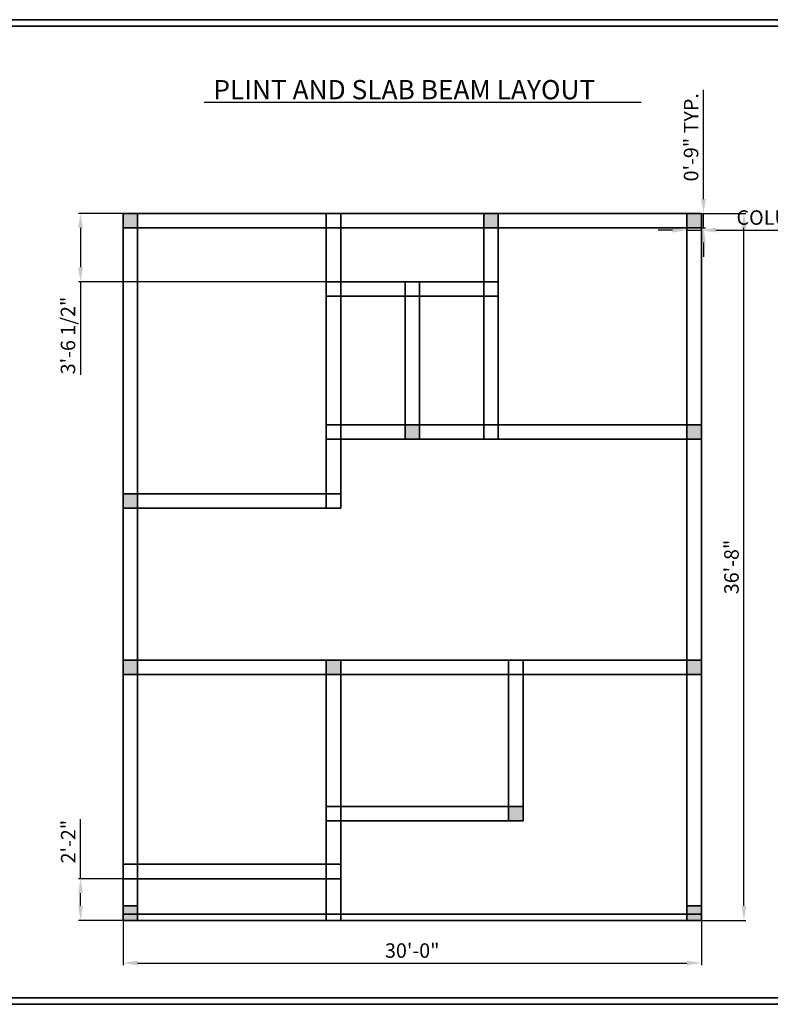
# Model space of a CAD drawing. Units: inches. Extents: x 2436 to 3928, y 1526 to 2149.
# Tile 5 of 6: x 2903 to 3371, y 1526 to 2138. Entities that reach past the tile are written whole.
import ezdxf

# ---------------------------------------------------------------- set-up
doc = ezdxf.new("R2010")
doc.units = ezdxf.units.IN
for name, color, linetype, lineweight in [('G-ANNO-TEXT', 7, 'Continuous', 25), ('G-ANNO-TTLB', 7, 'Continuous', 35), ('S-ANNO-DIMS', 2, 'Continuous', 18), ('S-BEAM', 7, 'Continuous', 35), ('S-COLS', 1, 'Continuous', 35), ('S-COLS-PATT', 1, 'Continuous', 13)]:
    doc.layers.add(name, color=color, linetype=linetype, lineweight=lineweight)
doc.styles.get("Standard").update_dxf_attribs({"font": 'arial.ttf'})
doc.dimstyles.new('ISO-25', dxfattribs={"dimtxt": 9, "dimasz": 9, "dimexe": 1.25, "dimexo": 0.625, "dimgap": 2, "dimtad": 1, "dimdec": 1, "dimlunit": 4, "dimtxsty": 'Standard', "dimcen": 2.5, "dimadec": 0, "dimazin": 0, "dimtfac": 1, "dimtdec": 1, "dimtmove": 0, "dimatfit": 3, "dimfxl": 1, "dimarcsym": 0})

# ---------------------------------------------------------------- blocks, each defined once
blk = doc.blocks.new('COL-9x9-PLAN')
h = blk.add_hatch(color=256)
h.dxf.hatch_style = 1
h.paths.add_polyline_path([(9, 0), (9, 9), (0, 9), (0, 0)])
blk.add_lwpolyline([(0, 9), (9, 9), (9, 0), (0, 0)], close=True)
blk = doc.blocks.new('*D30')
at = {"layer": 'Defpoints', "color": 0, "transparency": 16777216}
for p in [(3318.67, 2008.79), (3327.67, 2008.79), (3327.67, 2007.44)]:
    blk.add_point(p, dxfattribs=at)
at = {"layer": 'S-ANNO-DIMS', "color": 0, "lineweight": -2, "transparency": 16777216}
for p, q in [((3309.67, 2007.44), (3300.67, 2007.44)), ((3318.67, 2008.16), (3318.67, 2006.19)), ((3318.67, 2007.44), (3327.67, 2007.44)), ((3327.67, 2008.16), (3327.67, 2006.19)), ((3336.67, 2007.44), (3462.4, 2007.44))]:
    blk.add_line(p, q, dxfattribs=at)
at = {"layer": 'S-ANNO-DIMS', "color": 0, "transparency": 16777216}
for points in [[(3309.67, 2008.94), (3309.67, 2005.94), (3318.67, 2007.44)], [(3336.67, 2008.94), (3336.67, 2005.94), (3327.67, 2007.44)]]:
    blk.add_solid(points, dxfattribs=at)
at = {"layer": 'S-ANNO-DIMS', "color": 0, "transparency": 16777216, "insert": (3404.03, 2014.1), "char_height": 9, "attachment_point": 5}
blk.add_mtext('COLUMN 0\'-9" TYP.', dxfattribs=at)
blk = doc.blocks.new('*D31')
at = {"layer": 'Defpoints', "color": 0, "transparency": 16777216}
for p in [(3327.67, 2017.79), (3329.02, 2017.79), (3327.67, 2008.79)]:
    blk.add_point(p, dxfattribs=at)
at = {"layer": 'S-ANNO-DIMS', "color": 0, "lineweight": -2, "transparency": 16777216}
for p, q in [((3329.02, 2026.79), (3329.02, 2094.65)), ((3328.29, 2017.79), (3330.27, 2017.79)), ((3329.02, 2008.79), (3329.02, 2017.79)), ((3328.29, 2008.79), (3330.27, 2008.79)), ((3329.02, 1999.79), (3329.02, 1990.79))]:
    blk.add_line(p, q, dxfattribs=at)
at = {"layer": 'S-ANNO-DIMS', "color": 0, "transparency": 16777216}
for points in [[(3327.52, 2026.79), (3330.52, 2026.79), (3329.02, 2017.79)], [(3327.52, 1999.79), (3330.52, 1999.79), (3329.02, 2008.79)]]:
    blk.add_solid(points, dxfattribs=at)
at = {"layer": 'S-ANNO-DIMS', "color": 0, "transparency": 16777216, "insert": (3322.42, 2065.22), "char_height": 9, "attachment_point": 5, "rotation": 90}
blk.add_mtext('0\'-9" TYP.', dxfattribs=at)
blk = doc.blocks.new('*D74')
at = {"layer": 'Defpoints', "color": 0, "transparency": 16777216}
for p in [(2967.67, 1577.79), (3327.67, 1577.79), (3327.67, 1551.29)]:
    blk.add_point(p, dxfattribs=at)
at = {"layer": 'S-ANNO-DIMS', "color": 0, "lineweight": -2, "transparency": 16777216}
for p, q in [((2967.67, 1577.16), (2967.67, 1550.04)), ((3327.67, 1577.16), (3327.67, 1550.04)), ((2976.67, 1551.29), (3318.67, 1551.29))]:
    blk.add_line(p, q, dxfattribs=at)
at = {"layer": 'S-ANNO-DIMS', "color": 0, "transparency": 16777216}
for points in [[(2976.67, 1552.79), (2976.67, 1549.79), (2967.67, 1551.29)], [(3318.67, 1552.79), (3318.67, 1549.79), (3327.67, 1551.29)]]:
    blk.add_solid(points, dxfattribs=at)
at = {"layer": 'S-ANNO-DIMS', "color": 0, "transparency": 16777216, "insert": (3147.67, 1557.89), "char_height": 9, "attachment_point": 5}
blk.add_mtext('30\'-0"', dxfattribs=at)
blk = doc.blocks.new('*D75')
at = {"layer": 'Defpoints', "color": 0, "transparency": 16777216}
for p in [(3327.67, 2017.79), (3354.17, 2017.79), (3327.67, 1577.79)]:
    blk.add_point(p, dxfattribs=at)
at = {"layer": 'S-ANNO-DIMS', "color": 0, "lineweight": -2, "transparency": 16777216}
for p, q in [((3328.29, 2017.79), (3355.42, 2017.79)), ((3354.17, 1586.79), (3354.17, 2008.79)), ((3328.29, 1577.79), (3355.42, 1577.79))]:
    blk.add_line(p, q, dxfattribs=at)
at = {"layer": 'S-ANNO-DIMS', "color": 0, "transparency": 16777216}
for points in [[(3352.67, 2008.79), (3355.67, 2008.79), (3354.17, 2017.79)], [(3352.67, 1586.79), (3355.67, 1586.79), (3354.17, 1577.79)]]:
    blk.add_solid(points, dxfattribs=at)
at = {"layer": 'S-ANNO-DIMS', "color": 0, "transparency": 16777216, "insert": (3347.57, 1797.79), "char_height": 9, "attachment_point": 5, "rotation": 90}
blk.add_mtext('36\'-8"', dxfattribs=at)
blk = doc.blocks.new('*D76')
at = {"layer": 'Defpoints', "color": 0, "transparency": 16777216}
for p in [(3094.17, 2017.79), (2941.17, 1975.29), (3094.17, 1975.29)]:
    blk.add_point(p, dxfattribs=at)
at = {"layer": 'S-ANNO-DIMS', "color": 0, "lineweight": -2, "transparency": 16777216}
for p, q in [((3093.54, 2017.79), (2939.92, 2017.79)), ((2941.17, 2008.79), (2941.17, 1984.29)), ((3093.54, 1975.29), (2939.92, 1975.29)), ((2941.17, 1975.29), (2941.17, 1917.4))]:
    blk.add_line(p, q, dxfattribs=at)
at = {"layer": 'S-ANNO-DIMS', "color": 0, "transparency": 16777216}
for points in [[(2939.67, 2008.79), (2942.67, 2008.79), (2941.17, 2017.79)], [(2939.67, 1984.29), (2942.67, 1984.29), (2941.17, 1975.29)]]:
    blk.add_solid(points, dxfattribs=at)
at = {"layer": 'S-ANNO-DIMS', "color": 0, "transparency": 16777216, "insert": (2934.51, 1941.84), "char_height": 9, "attachment_point": 5, "rotation": 90}
blk.add_mtext('3\'-6 1/2"', dxfattribs=at)
blk = doc.blocks.new('*D77')
at = {"layer": 'Defpoints', "color": 0, "transparency": 16777216}
for p in [(2941.17, 1603.79), (2967.67, 1603.79), (2967.67, 1577.79)]:
    blk.add_point(p, dxfattribs=at)
at = {"layer": 'S-ANNO-DIMS', "color": 0, "lineweight": -2, "transparency": 16777216}
for p, q in [((2941.17, 1603.79), (2941.17, 1640.87)), ((2967.04, 1603.79), (2939.92, 1603.79)), ((2941.17, 1586.79), (2941.17, 1594.79)), ((2967.04, 1577.79), (2939.92, 1577.79))]:
    blk.add_line(p, q, dxfattribs=at)
at = {"layer": 'S-ANNO-DIMS', "color": 0, "transparency": 16777216}
for points in [[(2939.67, 1594.79), (2942.67, 1594.79), (2941.17, 1603.79)], [(2939.67, 1586.79), (2942.67, 1586.79), (2941.17, 1577.79)]]:
    blk.add_solid(points, dxfattribs=at)
at = {"layer": 'S-ANNO-DIMS', "color": 0, "transparency": 16777216, "insert": (2934.65, 1626.83), "char_height": 9, "attachment_point": 5, "rotation": 90}
blk.add_mtext('2\'-2"', dxfattribs=at)

msp = doc.modelspace()

# ---------------------------------------------------------------- hatches: boundary and pattern name
at = {"layer": 'S-COLS-PATT'}
h = msp.add_hatch(color=256, dxfattribs=at)
h.dxf.hatch_style = 1
h.paths.add_polyline_path([(3327.67, 1739.79), (3318.67, 1739.79), (3318.67, 1730.79), (3327.67, 1730.79)])

# ---------------------------------------------------------------- linework, layer by layer
at = {"layer": 'G-ANNO-TEXT'}
msp.add_line((3018.04, 2087.13), (3290.21, 2087.13), dxfattribs=at)
at = {"layer": 'G-ANNO-TTLB'}
for points in [[(2436, 2138.4), (3927.51, 2138.4), (3927.51, 1525.6), (2436, 1525.6)], [(2440, 2134.4), (3923.51, 2134.4), (3923.51, 1529.6), (2440, 1529.6)]]:
    msp.add_lwpolyline(points, close=True, dxfattribs=at)
at = {"layer": 'S-BEAM'}
for p, q in [((2967.67, 2017.79), (3096.67, 2017.79)), ((2967.67, 2017.79), (3327.67, 2017.79)), ((2967.67, 1577.79), (2967.67, 2017.79)), ((2976.67, 1840.79), (2976.67, 2017.79)), ((3094.17, 1834.29), (3094.17, 2017.79)), ((3096.67, 2017.79), (3100.67, 2017.79)), ((3100.67, 2017.79), (3194.67, 2017.79)), ((3103.17, 1966.29), (3103.17, 2017.79)), ((3192.17, 1966.29), (3192.17, 2017.79)), ((3194.67, 2017.79), (3198.67, 2017.79)), ((3201.17, 1877.29), (3201.17, 2017.79)), ((3318.67, 2017.79), (3327.67, 2017.79)), ((3318.67, 1883.79), (3318.67, 2017.79)), ((3327.67, 2017.79), (3327.67, 2008.79)), ((3327.67, 2017.79), (3327.67, 1888.79)), ((3327.67, 2017.79), (3327.67, 1577.79)), ((2967.67, 2008.79), (3096.67, 2008.79)), ((2976.67, 2008.79), (3194.67, 2008.79)), ((3103.17, 1834.29), (3103.17, 2008.79)), ((3192.17, 2008.79), (3327.67, 2008.79)), ((3192.17, 1877.29), (3192.17, 2008.79)), ((3094.17, 1975.29), (3201.17, 1975.29)), ((3143.17, 1877.29), (3143.17, 1975.29)), ((3152.17, 1877.29), (3152.17, 1975.29)), ((3094.17, 1966.29), (3201.17, 1966.29)), ((3096.67, 1966.29), (3145.67, 1966.29)), ((3094.17, 1886.29), (3327.67, 1886.29)), ((3318.67, 1739.79), (3318.67, 1883.79)), ((3094.17, 1877.29), (3327.67, 1877.29)), ((2967.67, 1843.29), (3103.17, 1843.29)), ((2976.67, 1739.79), (2976.67, 1840.79)), ((2967.67, 1834.29), (3103.17, 1834.29)), ((3327.67, 1744.79), (3327.67, 1732.79)), ((2967.67, 1739.79), (3327.67, 1739.79)), ((2976.67, 1739.79), (3064.67, 1739.79)), ((2976.67, 1603.79), (2976.67, 1739.79)), ((3094.17, 1577.79), (3094.17, 1739.79)), ((3103.17, 1577.79), (3103.17, 1739.79)), ((3207.67, 1639.79), (3207.67, 1739.79)), ((3216.67, 1639.79), (3216.67, 1739.79)), ((3316.67, 1739.79), (3318.67, 1739.79)), ((3318.67, 1577.79), (3318.67, 1739.79)), ((2967.67, 1730.79), (3327.67, 1730.79)), ((3327.67, 1732.79), (3327.67, 1577.79)), ((3216.67, 1648.79), (3094.17, 1648.79)), ((3094.17, 1639.79), (3216.67, 1639.79)), ((2967.67, 1612.79), (3103.17, 1612.79)), ((2967.67, 1603.79), (3103.17, 1603.79)), ((2967.67, 1577.79), (2967.67, 1603.79)), ((2976.67, 1581.79), (2976.67, 1603.79)), ((2967.67, 1581.79), (2967.67, 1595.79)), ((2967.67, 1581.79), (3327.67, 1581.79)), ((2967.67, 1577.79), (3327.67, 1577.79))]:
    msp.add_line(p, q, dxfattribs=at)
at = {"layer": 'S-COLS'}
msp.add_lwpolyline([(3318.67, 1739.79), (3327.67, 1739.79), (3327.67, 1730.79), (3318.67, 1730.79)], close=True, dxfattribs=at)

# ---------------------------------------------------------------- block references
for p in [(2967.67, 2008.79), (3192.17, 2008.79), (3318.67, 2008.79), (3143.17, 1877.29), (3318.67, 1877.29), (2967.67, 1834.29), (2967.67, 1730.79), (3094.17, 1730.79), (3207.67, 1639.79), (2967.67, 1577.79), (3318.67, 1577.79)]:
    msp.add_blockref('COL-9x9-PLAN', p, dxfattribs=at)

# ---------------------------------------------------------------- texts
at = {"layer": 'G-ANNO-TEXT'}
msp.add_text('PLINT AND SLAB BEAM LAYOUT', height=12, dxfattribs=at).set_placement((3023.84, 2088.86))

# ---------------------------------------------------------------- dimensions: what is measured, and where the dimension line sits
at = {"layer": 'S-ANNO-DIMS'}
dim = msp.add_linear_dim(base=(3329.02, 2017.79), p1=(3327.67, 2008.79), p2=(3327.67, 2017.79), angle=90, text='<> TYP.', dimstyle='ISO-25', override={"dimdec": 1, "dimlfac": 1, "dimrnd": 0, "dimzin": 1, "dimdsep": 46, "dimlunit": 4, "dimfrac": 2}, dxfattribs=at)
dim.commit()
dim.dimension.update_dxf_attribs({"geometry": '*D31', "text_midpoint": (3322.42, 2065.22)})
dim = msp.add_linear_dim(base=(3327.67, 2007.44), p1=(3318.67, 2008.79), p2=(3327.67, 2008.79), text='COLUMN <> TYP.', dimstyle='ISO-25', override={"dimdec": 1, "dimlfac": 1, "dimrnd": 0, "dimzin": 1, "dimdsep": 46, "dimlunit": 4, "dimfrac": 2}, dxfattribs=at)
dim.commit()
dim.dimension.update_dxf_attribs({"geometry": '*D30', "text_midpoint": (3404.03, 2014.1)})
for base, p1, p2, picture, middle in [((2941.17, 1975.29), (3094.17, 2017.79), (3094.17, 1975.29), '*D76', (2934.51, 1941.84)), ((3354.17, 2017.79), (3327.67, 1577.79), (3327.67, 2017.79), '*D75', (3347.57, 1797.79)), ((2941.17, 1603.79), (2967.67, 1577.79), (2967.67, 1603.79), '*D77', (2934.65, 1626.83))]:
    dim = msp.add_linear_dim(base=base, p1=p1, p2=p2, angle=90, dimstyle='ISO-25', override={"dimdec": 1, "dimlfac": 1, "dimrnd": 0, "dimzin": 1, "dimdsep": 46, "dimlunit": 4, "dimfrac": 2}, dxfattribs=at)
    dim.commit()
    dim.dimension.update_dxf_attribs({"geometry": picture, "text_midpoint": middle})
dim = msp.add_linear_dim(base=(3327.67, 1551.29), p1=(2967.67, 1577.79), p2=(3327.67, 1577.79), dimstyle='ISO-25', override={"dimdec": 1, "dimlfac": 1, "dimrnd": 0, "dimzin": 1, "dimdsep": 46, "dimlunit": 4, "dimfrac": 2}, dxfattribs=at)
dim.commit()
dim.dimension.update_dxf_attribs({"geometry": '*D74', "text_midpoint": (3147.67, 1557.89)})

doc.saveas('drawing.dxf')
